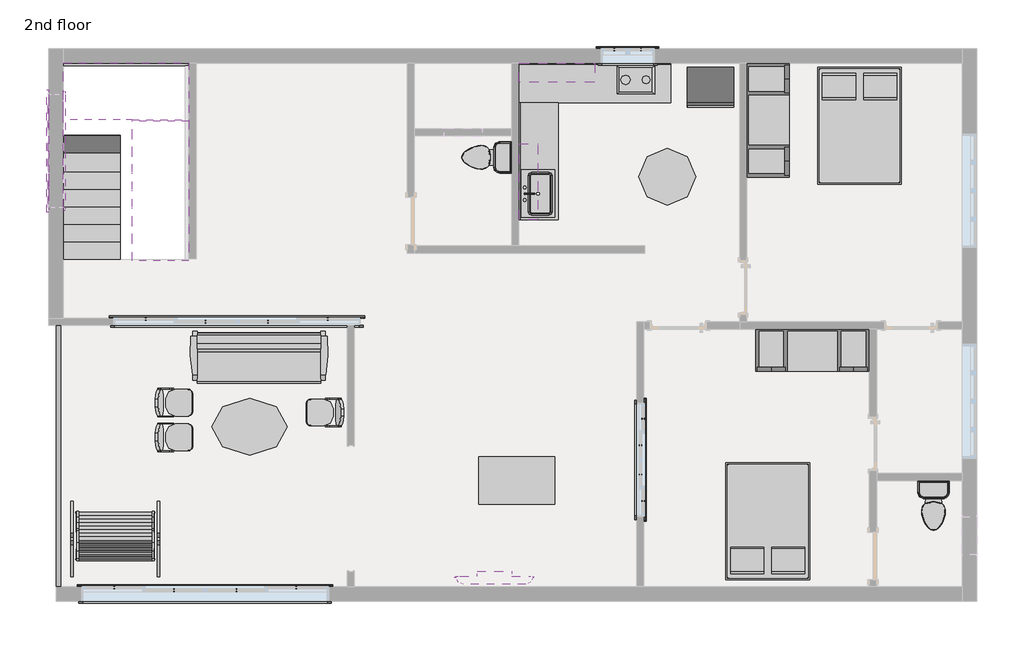
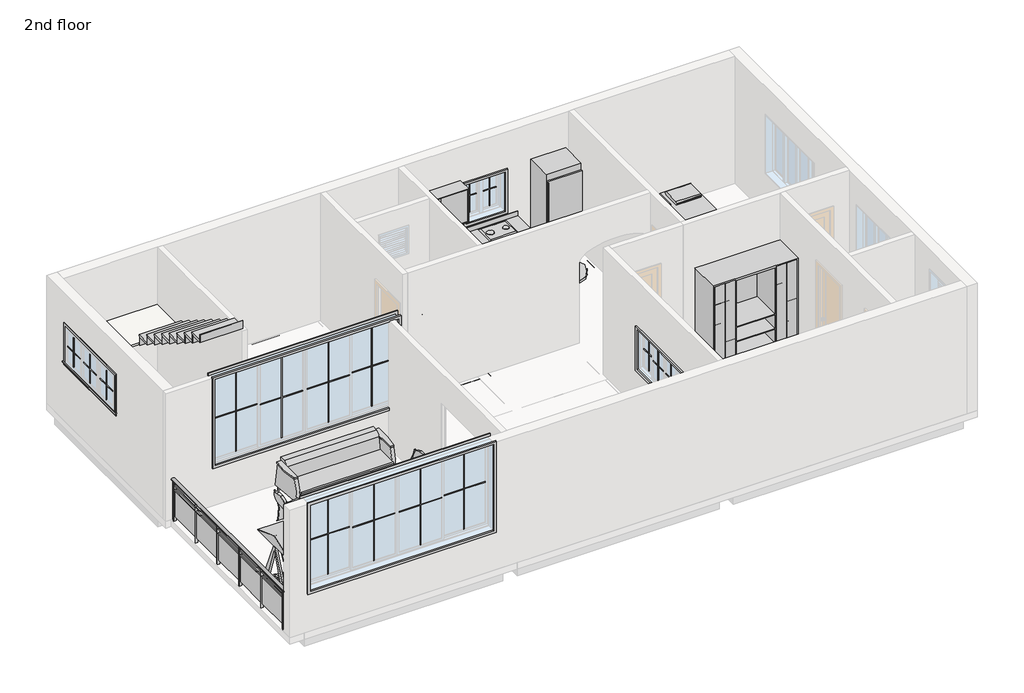
# One storey, part 2 of 2: 30 proxies, 21 furniture elements, 7 beams, 3 flow terminals, 2 stair flights, 1 railing, 1 slab.
"""IFC4 building model written with IfcOpenShell, lengths in millimetres."""

from ifc_helpers import new_model, si_unit, point, frame, origin, place, context, project, spatial, polyline, ellipse_curve, trimmed, outline, extrude, faceted_brep, transform, mapped, element, save
from ifc_brep_helpers import plane_surface, extruded_surface, advanced_brep
from components import proxy_3c1fa1d0, proxy_caef4acf, muntin_pattern_2x2_muntin_pattern_2x2_31a16349, muntin_pattern_2x2_muntin_pattern_2x2_a56fcb99, muntin_pattern_2x2_muntin_pattern_2x2_c58f38d7, muntin_pattern_2x2_muntin_pattern_2x2_b3fe6957, muntin_pattern_2x2_muntin_pattern_2x2_3e0ecaf2, muntin_pattern_2x2_muntin_pattern_2x2_51cb8927, proxy_19935bb1, trim_window_exterior_flat_with_sill_3c945769, trim_window_exterior_flat_with_sill_7b949e88, trim_window_exterior_flat_with_sill_41619996, trim_window_exterior_flat_with_sill_170b7f0e, trim_window_interior_flat_picture_frame_0edfbaa2, trim_window_interior_flat_picture_frame_687edbe0, trim_window_interior_flat_picture_frame_51c85655, trim_window_interior_flat_picture_frame_cc79b2fe, flow_terminal_4d548711, toilet_domestic_3d_toilet_domestic_3d_ba6479b0, toilet_domestic_3d_toilet_domestic_3d_30431060, furniture_0762_x_0762mm_a8fad5e2, furniture_f87f75a4, furniture_97fe820d, furniture_b58f7881, furniture_deb1c5d1, furniture_078eb3f3, furniture_88072bd9, furniture_eb3a3c23, furniture_4a9d42a7, furniture_0b81fedb, furniture_acc2807d, furniture_52f35bf4, furniture_b94c68a7, furniture_f491f192, non_monolithic_landing_4d8e9abd, stair_flight_485682bc, stair_flight_0c18b218

model = new_model("IFC4")

# Units and contexts
model_context = context("Model", 3, world=origin())
ifc_project = project(units=[si_unit("LENGTHUNIT", "METRE", prefix="MILLI")], contexts=[model_context])

# Site, building, storey
site = spatial("IfcSite", under=ifc_project)
building = spatial("IfcBuilding", under=site)
storey = spatial("IfcBuildingStorey", under=building, Name="2nd floor", Elevation=7010.4)

# Beams
placement = place(None, origin())
element("IfcBeam", 1, ObjectType="Concrete-Rectangular Beam", at=placement, inside=storey, context=model_context, shape_type="Brep", body=[
    faceted_brep([(-12643.368339, 9510.993496, 7010.4), (-12643.368339, 9282.393496, 7010.4), (-10681.218339, 9282.393496, 7010.4), (-10452.618339, 9282.393496, 7010.4), (-7176.018339, 9282.393496, 7010.4), (-6947.418339, 9282.393496, 7010.4), (-5499.618339, 9282.393496, 7010.4), (-5271.018339, 9282.393496, 7010.4), (-3492.916739, 9282.393496, 7010.4), (-3264.316739, 9282.393496, 7010.4), (-1842.018339, 9282.393496, 7010.4), (-1613.418339, 9282.393496, 7010.4), (1790.181661, 9282.393496, 7010.4), (1790.181661, 9510.993496, 7010.4), (-1575.318339, 9510.993496, 7010.4), (-1575.318339, 9320.493496, 7010.4), (-1880.118339, 9320.493496, 7010.4), (-1880.118339, 9510.993496, 7010.4), (-6909.318339, 9510.993496, 7010.4), (-6909.318339, 9320.493496, 7010.4), (-7214.118339, 9320.493496, 7010.4), (-7214.118339, 9510.993496, 7010.4), (-10414.518339, 9510.993496, 7010.4), (-10414.518339, 9320.493496, 7010.4), (-10719.318339, 9320.493496, 7010.4), (-10719.318339, 9510.993496, 7010.4), (-12643.368339, 9282.393496, 6705.6), (-10681.218339, 9282.393496, 6705.6), (-10452.618339, 9282.393496, 6705.6), (-7176.018339, 9282.393496, 6705.6), (-6947.418339, 9282.393496, 6705.6), (-5499.618339, 9282.393496, 6705.6), (-5271.018339, 9282.393496, 6705.6), (-3492.916739, 9282.393496, 6705.6), (-3264.316739, 9282.393496, 6705.6), (-1842.018339, 9282.393496, 6705.6), (-1613.418339, 9282.393496, 6705.6), (1790.181661, 9282.393496, 6705.6), (-12643.368339, 9510.993496, 6705.6), (-10719.318339, 9510.993496, 6705.6), (-10719.318339, 9320.493496, 6705.6), (-10414.518339, 9320.493496, 6705.6), (-10414.518339, 9510.993496, 6705.6), (-7214.118339, 9510.993496, 6705.6), (-7214.118339, 9320.493496, 6705.6), (-6909.318339, 9320.493496, 6705.6), (-6909.318339, 9510.993496, 6705.6), (-1880.118339, 9510.993496, 6705.6), (-1880.118339, 9320.493496, 6705.6), (-1575.318339, 9320.493496, 6705.6), (-1575.318339, 9510.993496, 6705.6), (1790.181661, 9510.993496, 6705.6)], [[[0, 1, 2, 3, 4, 5, 6, 7, 8, 9, 10, 11, 12, 13, 14, 15, 16, 17, 18, 19, 20, 21, 22, 23, 24, 25]], [[1, 26, 27, 28, 29, 30, 31, 32, 33, 34, 35, 36, 37, 12, 11, 10, 9, 8, 7, 6, 5, 4, 3, 2]], [[26, 38, 39, 40, 41, 42, 43, 44, 45, 46, 47, 48, 49, 50, 51, 37, 36, 35, 34, 33, 32, 31, 30, 29, 28, 27]], [[13, 51, 50, 14]], [[1, 0, 38, 26]], [[13, 12, 37, 51]], [[41, 23, 22, 42]], [[23, 41, 40, 24]], [[24, 40, 39, 25]], [[38, 0, 25, 39]], [[45, 19, 18, 46]], [[19, 45, 44, 20]], [[20, 44, 43, 21]], [[42, 22, 21, 43]], [[49, 15, 14, 50]], [[15, 49, 48, 16]], [[16, 48, 47, 17]], [[46, 18, 17, 47]]]),
])
element("IfcBeam", 2, ObjectType="Concrete-Rectangular Beam", at=placement, inside=storey, context=model_context, shape_type="Brep", body=[
    faceted_brep([(1790.181661, 913.093496, 7010.4), (2018.781661, 913.093496, 7010.4), (2018.781661, 4958.043496, 7010.4), (1790.181661, 4958.043496, 7010.4), (1790.181661, 2792.693496, 7010.4), (1790.181661, 2564.093496, 7010.4), (1790.181661, 913.093496, 6705.6), (1790.181661, 4958.043496, 6705.6), (1790.181661, 2792.693496, 6705.6), (1790.181661, 2564.093496, 6705.6), (2018.781661, 913.093496, 6705.6), (2018.781661, 4958.043496, 6705.6)], [[[0, 1, 2, 3, 4, 5]], [[6, 0, 5, 4, 3, 7, 8, 9]], [[10, 6, 9, 8, 7, 11]], [[1, 10, 11, 2]], [[1, 0, 6, 10]], [[3, 2, 11, 7]]]),
    faceted_brep([(1790.181661, 9244.293496, 7010.4), (2018.781661, 9244.293496, 7010.4), (2018.781661, 9244.293496, 6705.6), (1790.181661, 9244.293496, 6705.6), (2018.781661, 5262.843496, 7010.4), (1790.181661, 5262.843496, 7010.4), (1790.181661, 5262.843496, 6705.6), (2018.781661, 5262.843496, 6705.6), (1790.181661, 6289.4504179, 7010.4), (1790.181661, 6060.8155957, 7010.4), (1790.181661, 6289.4504179, 6705.6), (1790.181661, 6060.8155957, 6705.6)], [[[0, 1, 2, 3]], [[4, 5, 6, 7]], [[1, 0, 8, 9, 5, 4]], [[0, 3, 10, 11, 6, 5, 9, 8]], [[3, 2, 7, 6, 11, 10]], [[2, 1, 4, 7]]]),
])
element("IfcBeam", 3, ObjectType="Concrete-Rectangular Beam", at=placement, inside=storey, context=model_context, shape_type="SweptSolid", body=[
    extrude(outline(polyline([(-6947.418339, 8094.943496), (-6947.418339, 8323.543496), (-5499.618339, 8323.543496), (-5499.618339, 8094.943496), (-6947.418339, 8094.943496)])), frame((0.0, 0.0, 6705.6), z_axis=(0.0, 0.0, 1.0), x_axis=(1.0, 0.0, 0.0)), (0.0, 0.0, 1.0), 304.8),
])
element("IfcBeam", 4, ObjectType="Concrete-Rectangular Beam", at=placement, inside=storey, context=model_context, shape_type="Brep", body=[
    faceted_brep([(1790.181661, 6060.8155957, 7010.4), (1790.181661, 6289.4504179, 7010.4), (-1613.418339, 6348.8604768, 7010.4), (-1842.018339, 6352.8507047, 7010.4), (-3264.316739, 6377.6770156, 7010.4), (-3492.916739, 6381.6672435, 7010.4), (-5271.018339, 6412.7041223, 7010.4), (-5271.018339, 6184.0693001, 7010.4), (-3492.916739, 6153.0324213, 7010.4), (-3264.316739, 6149.0421934, 7010.4), (-1842.018339, 6124.2158825, 7010.4), (-1613.418339, 6120.2256547, 7010.4), (1790.181661, 6060.8155957, 6705.6), (-5271.018339, 6184.0693001, 6705.6), (-3492.916739, 6153.0324213, 6705.6), (-3264.316739, 6149.0421934, 6705.6), (-1842.018339, 6124.2158825, 6705.6), (-1613.418339, 6120.2256547, 6705.6), (1790.181661, 6289.4504179, 6705.6), (-5271.018339, 6412.7041223, 6705.6), (-3492.916739, 6381.6672435, 6705.6), (-3264.316739, 6377.6770156, 6705.6), (-1842.018339, 6352.8507047, 6705.6), (-1613.418339, 6348.8604768, 6705.6)], [[[0, 1, 2, 3, 4, 5, 6, 7, 8, 9, 10, 11]], [[12, 0, 11, 10, 9, 8, 7, 13, 14, 15, 16, 17]], [[18, 12, 17, 16, 15, 14, 13, 19, 20, 21, 22, 23]], [[1, 18, 23, 22, 21, 20, 19, 6, 5, 4, 3, 2]], [[1, 0, 12, 18]], [[7, 6, 19, 13]]]),
    faceted_brep([(-6947.418339, 6213.330971, 7010.4), (-6947.418339, 6441.9657932, 7010.4), (-6947.418339, 6441.9657932, 6705.6), (-6947.418339, 6213.330971, 6705.6), (-5499.618339, 6416.6943502, 7010.4), (-5499.618339, 6188.059528, 7010.4), (-5499.618339, 6188.059528, 6705.6), (-5499.618339, 6416.6943502, 6705.6)], [[[0, 1, 2, 3]], [[4, 5, 6, 7]], [[1, 0, 5, 4]], [[0, 3, 6, 5]], [[3, 2, 7, 6]], [[2, 1, 4, 7]]]),
])
element("IfcBeam", 5, ObjectType="Concrete-Rectangular Beam", at=placement, inside=storey, context=model_context, shape_type="Brep", body=[
    faceted_brep([(-1842.018339, 913.093496, 7010.4), (-1613.418339, 913.093496, 7010.4), (-1613.418339, 4996.143496, 7010.4), (-1613.418339, 5224.743496, 7010.4), (-1613.418339, 6120.2256547, 7010.4), (-1842.018339, 6124.2158825, 7010.4), (-1842.018339, 5281.893496, 7010.4), (-1784.868339, 5281.893496, 7010.4), (-1784.868339, 5053.293496, 7010.4), (-1842.018339, 5053.293496, 7010.4), (-1842.018339, 4996.143496, 7010.4), (-1842.018339, 913.093496, 6705.6), (-1842.018339, 5053.293496, 6705.6), (-1842.018339, 4996.143496, 6705.6), (-1613.418339, 913.093496, 6705.6), (-1784.868339, 5053.293496, 6705.6), (-1784.868339, 5281.893496, 6705.6), (-1842.018339, 5281.893496, 6705.6), (-1842.018339, 6124.2158825, 6705.6), (-1613.418339, 6120.2256547, 6705.6), (-1613.418339, 5224.743496, 6705.6), (-1613.418339, 4996.143496, 6705.6)], [[[0, 1, 2, 3, 4, 5, 6, 7, 8, 9, 10]], [[11, 0, 10, 9, 12, 13]], [[14, 11, 13, 12, 15, 16, 17, 18, 19, 20, 21]], [[1, 14, 21, 20, 19, 4, 3, 2]], [[1, 0, 11, 14]], [[5, 4, 19, 18]], [[8, 15, 12, 9]], [[16, 7, 6, 17]], [[7, 16, 15, 8]], [[5, 18, 17, 6]]]),
    faceted_brep([(-1842.018339, 9282.393496, 7010.4), (-1613.418339, 9282.393496, 7010.4), (-1613.418339, 9282.393496, 6705.6), (-1842.018339, 9282.393496, 6705.6), (-1613.418339, 6348.8604768, 7010.4), (-1842.018339, 6352.8507047, 7010.4), (-1842.018339, 6352.8507047, 6705.6), (-1613.418339, 6348.8604768, 6705.6)], [[[0, 1, 2, 3]], [[4, 5, 6, 7]], [[1, 0, 5, 4]], [[3, 2, 7, 6]], [[2, 1, 4, 7]], [[0, 3, 6, 5]]]),
])
element("IfcBeam", 6, ObjectType="Concrete-Rectangular Beam", at=placement, inside=storey, context=model_context, shape_type="Brep", body=[
    faceted_brep([(240.781661, 913.093496, 7010.4), (469.381661, 913.093496, 7010.4), (469.381661, 2564.093496, 7010.4), (469.381661, 2792.693496, 7010.4), (469.381661, 4996.143496, 7010.4), (240.781661, 4996.143496, 7010.4), (469.381661, 913.093496, 6705.6), (469.381661, 2564.093496, 6705.6), (469.381661, 2792.693496, 6705.6), (469.381661, 4996.143496, 6705.6), (240.781661, 913.093496, 6705.6), (240.781661, 4996.143496, 6705.6)], [[[0, 1, 2, 3, 4, 5]], [[1, 6, 7, 8, 9, 4, 3, 2]], [[6, 10, 11, 9, 8, 7]], [[10, 0, 5, 11]], [[1, 0, 10, 6]], [[5, 4, 9, 11]]]),
])
element("IfcBeam", 7, ObjectType="Concrete-Rectangular Beam", at=placement, inside=storey, context=model_context, shape_type="SweptSolid", body=[
    extrude(outline(polyline([(1790.181661, 2792.693496), (1790.181661, 2564.093496), (469.381661, 2564.093496), (469.381661, 2792.693496), (1790.181661, 2792.693496)])), frame((0.0, 0.0, 6705.6), z_axis=(0.0, 0.0, 1.0), x_axis=(1.0, 0.0, 0.0)), (0.0, 0.0, 1.0), 304.8),
])

# Proxies
proxy_shape = proxy_3c1fa1d0(model_context)
element("IfcBuildingElementProxy", 8, Name="Cook Top-2 Unit : 12\" x 18\"", ObjectType="Cook Top-2 Unit : 12\" x 18\"", at=placement, inside=storey, context=model_context, shape_type="MappedRepresentation", body=[
    mapped(proxy_shape, transform((-3421.5185434, 8977.593496, 7010.4), x_axis=(0.0, 1.0, 0.0), y_axis=(-1.0, 0.0, 0.0), z_axis=(0.0, 0.0, 1.0))),
])
proxy_2_shape = proxy_caef4acf(model_context)
element("IfcBuildingElementProxy", 9, Name="Cook Top-2 Unit : 16\" x 22\"", ObjectType="Cook Top-2 Unit : 16\" x 22\"", at=placement, inside=storey, context=model_context, shape_type="MappedRepresentation", body=[
    mapped(proxy_2_shape, transform((-3370.7185434, 8977.593496, 7010.4), x_axis=(0.0, 1.0, 0.0), y_axis=(-1.0, 0.0, 0.0), z_axis=(0.0, 0.0, 1.0))),
])
muntin_pattern_2x2_muntin_pattern_2x2_shape = muntin_pattern_2x2_muntin_pattern_2x2_31a16349(model_context)
element("IfcBuildingElementProxy", 10, Name="Muntin Pattern_2x2 : Muntin Pattern_2x2", ObjectType="Muntin Pattern_2x2 : Muntin Pattern_2x2", at=placement, inside=storey, context=model_context, shape_type="MappedRepresentation", body=[
    mapped(muntin_pattern_2x2_muntin_pattern_2x2_shape, transform((-3330.991739, 3615.018496, 8007.35), x_axis=(0.0, -1.0, 0.0), y_axis=(1.0, 0.0, 0.0), z_axis=(0.0, 0.0, 1.0))),
])
element("IfcBuildingElementProxy", 11, Name="Muntin Pattern_2x2 : Muntin Pattern_2x2", ObjectType="Muntin Pattern_2x2 : Muntin Pattern_2x2", at=placement, inside=storey, context=model_context, shape_type="MappedRepresentation", body=[
    mapped(muntin_pattern_2x2_muntin_pattern_2x2_shape, transform((-3375.441739, 3189.568496, 8007.35), x_axis=(0.0, -1.0, 0.0), y_axis=(1.0, 0.0, 0.0), z_axis=(0.0, 0.0, 1.0))),
])
element("IfcBuildingElementProxy", 12, Name="Muntin Pattern_2x2 : Muntin Pattern_2x2", ObjectType="Muntin Pattern_2x2 : Muntin Pattern_2x2", at=placement, inside=storey, context=model_context, shape_type="MappedRepresentation", body=[
    mapped(muntin_pattern_2x2_muntin_pattern_2x2_shape, transform((-3375.441739, 2719.668496, 8007.35), x_axis=(0.0, -1.0, 0.0), y_axis=(1.0, 0.0, 0.0), z_axis=(0.0, 0.0, 1.0))),
])
element("IfcBuildingElementProxy", 13, Name="Muntin Pattern_2x2 : Muntin Pattern_2x2", ObjectType="Muntin Pattern_2x2 : Muntin Pattern_2x2", at=placement, inside=storey, context=model_context, shape_type="MappedRepresentation", body=[
    mapped(muntin_pattern_2x2_muntin_pattern_2x2_shape, transform((-3330.991739, 2294.218496, 8007.35), x_axis=(0.0, -1.0, 0.0), y_axis=(1.0, 0.0, 0.0), z_axis=(0.0, 0.0, 1.0))),
])
muntin_pattern_2x2_muntin_pattern_2x2_2_shape = muntin_pattern_2x2_muntin_pattern_2x2_a56fcb99(model_context)
element("IfcBuildingElementProxy", 14, Name="Muntin Pattern_2x2 : Muntin Pattern_2x2", ObjectType="Muntin Pattern_2x2 : Muntin Pattern_2x2", at=placement, inside=storey, context=model_context, shape_type="MappedRepresentation", body=[
    mapped(muntin_pattern_2x2_muntin_pattern_2x2_2_shape, transform((-12862.443339, 7303.3101627, 8451.85), x_axis=(0.0, 1.0, 0.0), y_axis=(-1.0, 0.0, 0.0), z_axis=(0.0, 0.0, 1.0))),
])
element("IfcBuildingElementProxy", 15, Name="Muntin Pattern_2x2 : Muntin Pattern_2x2", ObjectType="Muntin Pattern_2x2 : Muntin Pattern_2x2", at=placement, inside=storey, context=model_context, shape_type="MappedRepresentation", body=[
    mapped(muntin_pattern_2x2_muntin_pattern_2x2_2_shape, transform((-12862.443339, 7910.793496, 8451.85), x_axis=(0.0, 1.0, 0.0), y_axis=(-1.0, 0.0, 0.0), z_axis=(0.0, 0.0, 1.0))),
])
muntin_pattern_2x2_muntin_pattern_2x2_3_shape = muntin_pattern_2x2_muntin_pattern_2x2_c58f38d7(model_context)
element("IfcBuildingElementProxy", 16, Name="Muntin Pattern_2x2 : Muntin Pattern_2x2", ObjectType="Muntin Pattern_2x2 : Muntin Pattern_2x2", at=placement, inside=storey, context=model_context, shape_type="MappedRepresentation", body=[
    mapped(muntin_pattern_2x2_muntin_pattern_2x2_3_shape, transform((-12862.443339, 8518.2768293, 8451.85), x_axis=(0.0, -1.0, 0.0), y_axis=(1.0, 0.0, 0.0), z_axis=(0.0, 0.0, 1.0))),
])
muntin_pattern_2x2_muntin_pattern_2x2_4_shape = muntin_pattern_2x2_muntin_pattern_2x2_b3fe6957(model_context)
element("IfcBuildingElementProxy", 17, Name="Muntin Pattern_2x2 : Muntin Pattern_2x2", ObjectType="Muntin Pattern_2x2 : Muntin Pattern_2x2", at=placement, inside=storey, context=model_context, shape_type="MappedRepresentation", body=[
    mapped(muntin_pattern_2x2_muntin_pattern_2x2_4_shape, transform((-3796.230839, 9539.568496, 8185.15), x_axis=(1.0, 0.0, 0.0), y_axis=(0.0, 1.0, 0.0), z_axis=(0.0, 0.0, 1.0))),
])
muntin_pattern_2x2_muntin_pattern_2x2_5_shape = muntin_pattern_2x2_muntin_pattern_2x2_3e0ecaf2(model_context)
element("IfcBuildingElementProxy", 18, Name="Muntin Pattern_2x2 : Muntin Pattern_2x2", ObjectType="Muntin Pattern_2x2 : Muntin Pattern_2x2", at=placement, inside=storey, context=model_context, shape_type="MappedRepresentation", body=[
    mapped(muntin_pattern_2x2_muntin_pattern_2x2_5_shape, transform((-3367.605839, 9539.568496, 8185.15), x_axis=(-1.0, 0.0, 0.0), y_axis=(0.0, -1.0, 0.0), z_axis=(0.0, 0.0, 1.0))),
])
muntin_pattern_2x2_muntin_pattern_2x2_6_shape = muntin_pattern_2x2_muntin_pattern_2x2_51cb8927(model_context)
element("IfcBuildingElementProxy", 19, Name="Muntin Pattern_2x2 : Muntin Pattern_2x2", ObjectType="Muntin Pattern_2x2 : Muntin Pattern_2x2", at=placement, inside=storey, context=model_context, shape_type="MappedRepresentation", body=[
    mapped(muntin_pattern_2x2_muntin_pattern_2x2_6_shape, transform((-11316.218339, 5215.218496, 8007.35), x_axis=(1.0, 0.0, 0.0), y_axis=(0.0, 1.0, 0.0), z_axis=(0.0, 0.0, 1.0))),
])
element("IfcBuildingElementProxy", 20, Name="Muntin Pattern_2x2 : Muntin Pattern_2x2", ObjectType="Muntin Pattern_2x2 : Muntin Pattern_2x2", at=placement, inside=storey, context=model_context, shape_type="MappedRepresentation", body=[
    mapped(muntin_pattern_2x2_muntin_pattern_2x2_6_shape, transform((-10357.368339, 5170.768496, 8007.35), x_axis=(1.0, 0.0, 0.0), y_axis=(0.0, 1.0, 0.0), z_axis=(0.0, 0.0, 1.0))),
])
element("IfcBuildingElementProxy", 21, Name="Muntin Pattern_2x2 : Muntin Pattern_2x2", ObjectType="Muntin Pattern_2x2 : Muntin Pattern_2x2", at=placement, inside=storey, context=model_context, shape_type="MappedRepresentation", body=[
    mapped(muntin_pattern_2x2_muntin_pattern_2x2_6_shape, transform((-9354.068339, 5170.768496, 8007.35), x_axis=(1.0, 0.0, 0.0), y_axis=(0.0, 1.0, 0.0), z_axis=(0.0, 0.0, 1.0))),
])
element("IfcBuildingElementProxy", 22, Name="Muntin Pattern_2x2 : Muntin Pattern_2x2", ObjectType="Muntin Pattern_2x2 : Muntin Pattern_2x2", at=placement, inside=storey, context=model_context, shape_type="MappedRepresentation", body=[
    mapped(muntin_pattern_2x2_muntin_pattern_2x2_6_shape, transform((-8395.218339, 5215.218496, 8007.35), x_axis=(1.0, 0.0, 0.0), y_axis=(0.0, 1.0, 0.0), z_axis=(0.0, 0.0, 1.0))),
])
element("IfcBuildingElementProxy", 23, Name="Muntin Pattern_2x2 : Muntin Pattern_2x2", ObjectType="Muntin Pattern_2x2 : Muntin Pattern_2x2", at=placement, inside=storey, context=model_context, shape_type="MappedRepresentation", body=[
    mapped(muntin_pattern_2x2_muntin_pattern_2x2_6_shape, transform((-11824.218339, 903.568496, 8007.35), x_axis=(1.0, 0.0, 0.0), y_axis=(0.0, 1.0, 0.0), z_axis=(0.0, 0.0, 1.0))),
])
element("IfcBuildingElementProxy", 24, Name="Muntin Pattern_2x2 : Muntin Pattern_2x2", ObjectType="Muntin Pattern_2x2 : Muntin Pattern_2x2", at=placement, inside=storey, context=model_context, shape_type="MappedRepresentation", body=[
    mapped(muntin_pattern_2x2_muntin_pattern_2x2_6_shape, transform((-10865.368339, 859.118496, 8007.35), x_axis=(1.0, 0.0, 0.0), y_axis=(0.0, 1.0, 0.0), z_axis=(0.0, 0.0, 1.0))),
])
element("IfcBuildingElementProxy", 25, Name="Muntin Pattern_2x2 : Muntin Pattern_2x2", ObjectType="Muntin Pattern_2x2 : Muntin Pattern_2x2", at=placement, inside=storey, context=model_context, shape_type="MappedRepresentation", body=[
    mapped(muntin_pattern_2x2_muntin_pattern_2x2_6_shape, transform((-9862.068339, 859.118496, 8007.35), x_axis=(1.0, 0.0, 0.0), y_axis=(0.0, 1.0, 0.0), z_axis=(0.0, 0.0, 1.0))),
])
element("IfcBuildingElementProxy", 26, Name="Muntin Pattern_2x2 : Muntin Pattern_2x2", ObjectType="Muntin Pattern_2x2 : Muntin Pattern_2x2", at=placement, inside=storey, context=model_context, shape_type="MappedRepresentation", body=[
    mapped(muntin_pattern_2x2_muntin_pattern_2x2_6_shape, transform((-8903.218339, 903.568496, 8007.35), x_axis=(1.0, 0.0, 0.0), y_axis=(0.0, 1.0, 0.0), z_axis=(0.0, 0.0, 1.0))),
])
proxy_3_shape = proxy_19935bb1(model_context)
element("IfcBuildingElementProxy", 27, Name="Refrigerator-Built-in : 30\" x 24\" LH", ObjectType="Refrigerator-Built-in : 30\" x 24\" LH", at=placement, inside=storey, context=model_context, shape_type="MappedRepresentation", body=[
    mapped(proxy_3_shape, transform((-2254.768339, 8966.8695245, 7010.4), x_axis=(1.0, 0.0, 0.0), y_axis=(0.0, 1.0, 0.0), z_axis=(0.0, 0.0, 1.0))),
])
trim_window_exterior_flat_with_sill_shape = trim_window_exterior_flat_with_sill_3c945769(model_context)
element("IfcBuildingElementProxy", 28, Name="Trim-Window-Exterior-Flat : with Sill", ObjectType="Trim-Window-Exterior-Flat : with Sill", at=placement, inside=storey, context=model_context, shape_type="MappedRepresentation", body=[
    mapped(trim_window_exterior_flat_with_sill_shape, transform((-3321.466739, 2954.618496, 8839.2), x_axis=(0.0, 1.0, 0.0), y_axis=(0.0, 0.0, 1.0), z_axis=(1.0, 0.0, 0.0))),
])
trim_window_exterior_flat_with_sill_2_shape = trim_window_exterior_flat_with_sill_7b949e88(model_context)
element("IfcBuildingElementProxy", 29, Name="Trim-Window-Exterior-Flat : with Sill", ObjectType="Trim-Window-Exterior-Flat : with Sill", at=placement, inside=storey, context=model_context, shape_type="MappedRepresentation", body=[
    mapped(trim_window_exterior_flat_with_sill_2_shape, transform((-12871.968339, 7910.793496, 9194.8), x_axis=(0.0, 1.0, 0.0), y_axis=(0.0, 0.0, -1.0), z_axis=(-1.0, 0.0, 0.0))),
])
trim_window_exterior_flat_with_sill_3_shape = trim_window_exterior_flat_with_sill_41619996(model_context)
element("IfcBuildingElementProxy", 30, Name="Trim-Window-Exterior-Flat : with Sill", ObjectType="Trim-Window-Exterior-Flat : with Sill", at=placement, inside=storey, context=model_context, shape_type="MappedRepresentation", body=[
    mapped(trim_window_exterior_flat_with_sill_3_shape, transform((-3581.918339, 9549.093496, 9029.7), x_axis=(-1.0, 0.0, 0.0), y_axis=(0.0, 0.0, 1.0), z_axis=(0.0, 1.0, 0.0))),
])
trim_window_exterior_flat_with_sill_4_shape = trim_window_exterior_flat_with_sill_170b7f0e(model_context)
element("IfcBuildingElementProxy", 31, Name="Trim-Window-Exterior-Flat : with Sill", ObjectType="Trim-Window-Exterior-Flat : with Sill", at=placement, inside=storey, context=model_context, shape_type="MappedRepresentation", body=[
    mapped(trim_window_exterior_flat_with_sill_4_shape, transform((-9855.718339, 5224.743496, 9906.0), x_axis=(-1.0, 0.0, 0.0), y_axis=(0.0, 0.0, 1.0), z_axis=(0.0, 1.0, 0.0))),
])
element("IfcBuildingElementProxy", 32, Name="Trim-Window-Exterior-Flat : with Sill", ObjectType="Trim-Window-Exterior-Flat : with Sill", at=placement, inside=storey, context=model_context, shape_type="MappedRepresentation", body=[
    mapped(trim_window_exterior_flat_with_sill_4_shape, transform((-10363.718339, 913.093496, 9906.0), x_axis=(-1.0, 0.0, 0.0), y_axis=(0.0, 0.0, 1.0), z_axis=(0.0, 1.0, 0.0))),
])
trim_window_interior_flat_picture_frame_shape = trim_window_interior_flat_picture_frame_0edfbaa2(model_context)
element("IfcBuildingElementProxy", 33, Name="Trim-Window-Interior-Flat : Picture Frame", ObjectType="Trim-Window-Interior-Flat : Picture Frame", at=placement, inside=storey, context=model_context, shape_type="MappedRepresentation", body=[
    mapped(trim_window_interior_flat_picture_frame_shape, transform((-3435.766739, 2954.618496, 8839.2), x_axis=(0.0, -1.0, 0.0), y_axis=(0.0, 0.0, 1.0), z_axis=(-1.0, 0.0, 0.0))),
])
trim_window_interior_flat_picture_frame_2_shape = trim_window_interior_flat_picture_frame_687edbe0(model_context)
element("IfcBuildingElementProxy", 34, Name="Trim-Window-Interior-Flat : Picture Frame", ObjectType="Trim-Window-Interior-Flat : Picture Frame", at=placement, inside=storey, context=model_context, shape_type="MappedRepresentation", body=[
    mapped(trim_window_interior_flat_picture_frame_2_shape, transform((-12643.368339, 7910.793496, 9194.8), x_axis=(0.0, -1.0, 0.0), y_axis=(0.0, 0.0, -1.0), z_axis=(1.0, 0.0, 0.0))),
])
trim_window_interior_flat_picture_frame_3_shape = trim_window_interior_flat_picture_frame_51c85655(model_context)
element("IfcBuildingElementProxy", 35, Name="Trim-Window-Interior-Flat : Picture Frame", ObjectType="Trim-Window-Interior-Flat : Picture Frame", at=placement, inside=storey, context=model_context, shape_type="MappedRepresentation", body=[
    mapped(trim_window_interior_flat_picture_frame_3_shape, transform((-3581.918339, 9320.493496, 9029.7), x_axis=(1.0, 0.0, 0.0), y_axis=(0.0, 0.0, 1.0), z_axis=(0.0, -1.0, 0.0))),
])
trim_window_interior_flat_picture_frame_4_shape = trim_window_interior_flat_picture_frame_cc79b2fe(model_context)
element("IfcBuildingElementProxy", 36, Name="Trim-Window-Interior-Flat : Picture Frame", ObjectType="Trim-Window-Interior-Flat : Picture Frame", at=placement, inside=storey, context=model_context, shape_type="MappedRepresentation", body=[
    mapped(trim_window_interior_flat_picture_frame_4_shape, transform((-9855.718339, 5110.443496, 9906.0), x_axis=(1.0, 0.0, 0.0), y_axis=(0.0, 0.0, 1.0), z_axis=(0.0, -1.0, 0.0))),
])
element("IfcBuildingElementProxy", 37, Name="Trim-Window-Interior-Flat : Picture Frame", ObjectType="Trim-Window-Interior-Flat : Picture Frame", at=placement, inside=storey, context=model_context, shape_type="MappedRepresentation", body=[
    mapped(trim_window_interior_flat_picture_frame_4_shape, transform((-10363.718339, 684.493496, 9906.0), x_axis=(1.0, 0.0, 0.0), y_axis=(0.0, 0.0, 1.0), z_axis=(0.0, -1.0, 0.0))),
])

# Flow terminals
flow_terminal_shape = flow_terminal_4d548711(model_context)
element("IfcFlowTerminal", 38, ObjectType="Sink Kitchen-Single : 30\" x 21\"", at=placement, inside=storey, context=model_context, shape_type="MappedRepresentation", body=[
    mapped(flow_terminal_shape, transform((-5021.0229378, 7209.3042554, 7010.4), x_axis=(0.0, 1.0, 0.0), y_axis=(-1.0, 0.0, 0.0), z_axis=(0.0, 0.0, 1.0))),
])
toilet_domestic_3d_toilet_domestic_3d_shape = toilet_domestic_3d_toilet_domestic_3d_ba6479b0(model_context)
toilet_domestic_3d_toilet_domestic_3d_2_shape = toilet_domestic_3d_toilet_domestic_3d_30431060(model_context)
element("IfcFlowTerminal", 39, ObjectType="Toilet-Domestic-3D : Toilet-Domestic-3D", at=placement, inside=storey, context=model_context, shape_type="MappedRepresentation", body=[
    mapped(toilet_domestic_3d_toilet_domestic_3d_shape, transform((-5937.1643663, 7809.6710196, 7010.4), x_axis=(0.0, -1.0, 0.0), y_axis=(1.0, 0.0, 0.0), z_axis=(0.0, 0.0, 1.0))),
    mapped(toilet_domestic_3d_toilet_domestic_3d_2_shape, transform((-5937.1643663, 7809.6710196, 7010.4), x_axis=(0.0, -1.0, 0.0), y_axis=(1.0, 0.0, 0.0), z_axis=(0.0, 0.0, 1.0))),
])
element("IfcFlowTerminal", 40, ObjectType="Toilet-Domestic-3D : Toilet-Domestic-3D", at=placement, inside=storey, context=model_context, shape_type="MappedRepresentation", body=[
    mapped(toilet_domestic_3d_toilet_domestic_3d_shape, transform((1325.531896, 2126.5474686, 7010.4), x_axis=(1.0, 0.0, 0.0), y_axis=(0.0, 1.0, 0.0), z_axis=(0.0, 0.0, 1.0))),
    mapped(toilet_domestic_3d_toilet_domestic_3d_2_shape, transform((1325.531896, 2126.5474686, 7010.4), x_axis=(1.0, 0.0, 0.0), y_axis=(0.0, 1.0, 0.0), z_axis=(0.0, 0.0, 1.0))),
])

# Furniture
furniture_0762_x_0762mm_shape = furniture_0762_x_0762mm_a8fad5e2(model_context)
element("IfcFurniture", 41, ObjectType="0762 x 0762mm", at=placement, inside=storey, context=model_context, shape_type="MappedRepresentation", body=[
    mapped(furniture_0762_x_0762mm_shape, transform((-11368.6588951, 2598.8675531, 7010.4), x_axis=(-1.0, 0.0, 0.0), y_axis=(0.0, -1.0, 0.0), z_axis=(0.0, 0.0, 1.0))),
])
furniture_shape = furniture_f87f75a4(model_context)
element("IfcFurniture", 42, ObjectType="Base Cabinet-Combo01 : 30\"", at=placement, inside=storey, context=model_context, shape_type="MappedRepresentation", body=[
    mapped(furniture_shape, transform((-4051.5060439, 9320.493496, 7010.4), x_axis=(1.0, 0.0, 0.0), y_axis=(0.0, 1.0, 0.0), z_axis=(0.0, 0.0, 1.0))),
])
element("IfcFurniture", 43, ObjectType="Base Cabinet-Combo01 : 30\"", at=placement, inside=storey, context=model_context, shape_type="MappedRepresentation", body=[
    mapped(furniture_shape, transform((-5328.168339, 8006.3557911, 7010.4), x_axis=(0.0, 1.0, 0.0), y_axis=(-1.0, 0.0, 0.0), z_axis=(0.0, 0.0, 1.0))),
])
element("IfcFurniture", 44, ObjectType="Base Cabinet-Combo01 : 30\"", at=placement, inside=storey, context=model_context, shape_type="MappedRepresentation", body=[
    mapped(furniture_shape, transform((-3289.5060439, 9320.493496, 7010.4), x_axis=(1.0, 0.0, 0.0), y_axis=(0.0, 1.0, 0.0), z_axis=(0.0, 0.0, 1.0))),
])
furniture_2_shape = furniture_97fe820d(model_context)
element("IfcFurniture", 45, ObjectType="Base Cabinet-Corner Unit-Square : 36\"", at=placement, inside=storey, context=model_context, shape_type="MappedRepresentation", body=[
    mapped(furniture_2_shape, transform((-5328.168339, 8793.7557911, 7010.4), x_axis=(0.0, 1.0, 0.0), y_axis=(-1.0, 0.0, 0.0), z_axis=(0.0, 0.0, 1.0))),
])
furniture_3_shape = furniture_b58f7881(model_context)
element("IfcFurniture", 46, ObjectType="Bed-Box : Double 53\" x 74\"", at=placement, inside=storey, context=model_context, shape_type="MappedRepresentation", body=[
    mapped(furniture_3_shape, transform((-199.970798, 8551.6230042, 7010.4), x_axis=(1.0, 0.0, 0.0), y_axis=(0.0, 1.0, 0.0), z_axis=(0.0, 0.0, 1.0))),
])
element("IfcFurniture", 47, ObjectType="Bed-Box : Double 53\" x 74\"", at=placement, inside=storey, context=model_context, shape_type="MappedRepresentation", body=[
    mapped(furniture_3_shape, transform((-994.7642799, 1732.7639878, 7010.4), x_axis=(-1.0, 0.0, 0.0), y_axis=(0.0, -1.0, 0.0), z_axis=(0.0, 0.0, 1.0))),
])
furniture_4_shape = furniture_deb1c5d1(model_context)
element("IfcFurniture", 48, ObjectType="Counter Top : 24\" Depth", at=placement, inside=storey, context=model_context, shape_type="MappedRepresentation", body=[
    mapped(furniture_4_shape, transform((-4127.7060439, 9320.493496, 7010.4), x_axis=(1.0, 0.0, 0.0), y_axis=(0.0, 1.0, 0.0), z_axis=(0.0, 0.0, 1.0))),
])
furniture_5_shape = furniture_078eb3f3(model_context)
element("IfcFurniture", 49, ObjectType="Counter Top w Sink Hole : 24\" Depth", at=placement, inside=storey, context=model_context, shape_type="MappedRepresentation", body=[
    mapped(furniture_5_shape, transform((-5328.168339, 8006.6364215, 7010.4), x_axis=(0.0, 1.0, 0.0), y_axis=(-1.0, 0.0, 0.0), z_axis=(0.0, 0.0, 1.0))),
])
furniture_6_shape = furniture_88072bd9(model_context)
element("IfcFurniture", 50, ObjectType="Entertainment Center.0001 : 72\" x 72\" x 24\"", at=placement, inside=storey, context=model_context, shape_type="MappedRepresentation", body=[
    mapped(furniture_6_shape, transform((-616.468339, 5154.893496, 7010.4), x_axis=(1.0, 0.0, 0.0), y_axis=(0.0, 1.0, 0.0), z_axis=(0.0, 0.0, 1.0))),
])
element("IfcFurniture", 51, ObjectType="Entertainment Center.0001 : 72\" x 72\" x 24\"", at=placement, inside=storey, context=model_context, shape_type="MappedRepresentation", body=[
    mapped(furniture_6_shape, transform((-1772.168339, 8406.093496, 7010.4), x_axis=(0.0, 1.0, 0.0), y_axis=(-1.0, 0.0, 0.0), z_axis=(0.0, 0.0, 1.0))),
])
furniture_7_shape = furniture_eb3a3c23(model_context)
element("IfcFurniture", 52, ObjectType="Seating-Auditorium : 18\" x 24\" x 30\"", at=placement, inside=storey, context=model_context, shape_type="MappedRepresentation", body=[
    mapped(furniture_7_shape, transform((-8243.4429291, 3552.7156271, 7010.4), x_axis=(0.0, 1.0, 0.0), y_axis=(-1.0, 0.0, 0.0), z_axis=(0.0, 0.0, 1.0))),
])
element("IfcFurniture", 53, ObjectType="Seating-Auditorium : 18\" x 24\" x 30\"", at=placement, inside=storey, context=model_context, shape_type="MappedRepresentation", body=[
    mapped(furniture_7_shape, transform((-11061.5937488, 3474.1213649, 7010.4), x_axis=(0.0, -1.0, 0.0), y_axis=(1.0, 0.0, 0.0), z_axis=(0.0, 0.0, 1.0))),
])
element("IfcFurniture", 54, ObjectType="Seating-Auditorium : 18\" x 24\" x 30\"", at=placement, inside=storey, context=model_context, shape_type="MappedRepresentation", body=[
    mapped(furniture_7_shape, transform((-11061.5937488, 4032.9213649, 7010.4), x_axis=(0.0, -1.0, 0.0), y_axis=(1.0, 0.0, 0.0), z_axis=(0.0, 0.0, 1.0))),
])
furniture_8_shape = furniture_4a9d42a7(model_context)
element("IfcFurniture", 55, ObjectType="Sofa-Pensi : 84\"", at=placement, inside=storey, context=model_context, shape_type="MappedRepresentation", body=[
    mapped(furniture_8_shape, transform((-9778.724589, 4325.3336599, 7010.4), x_axis=(1.0, 0.0, 0.0), y_axis=(0.0, 1.0, 0.0), z_axis=(0.0, 0.0, 1.0))),
])
furniture_9_shape = furniture_0b81fedb(model_context)
element("IfcFurniture", 56, ObjectType="TV - Flat Screen : 50\"", at=placement, inside=storey, context=model_context, shape_type="MappedRepresentation", body=[
    mapped(furniture_9_shape, transform((-5725.8128531, 1013.6142575, 8229.6), x_axis=(-1.0, 0.0, 0.0), y_axis=(0.0, -1.0, 0.0), z_axis=(0.0, 0.0, 1.0))),
])
furniture_10_shape = furniture_acc2807d(model_context)
element("IfcFurniture", 57, ObjectType="Table-Coffee Rectangular : 48\" x 30\"", at=placement, inside=storey, context=model_context, shape_type="MappedRepresentation", body=[
    mapped(furniture_10_shape, transform((-5973.1503692, 2251.6326642, 7010.4), x_axis=(1.0, 0.0, 0.0), y_axis=(0.0, 1.0, 0.0), z_axis=(0.0, 0.0, 1.0))),
])
furniture_11_shape = furniture_52f35bf4(model_context)
element("IfcFurniture", 58, ObjectType="Table-Dining Round w Chairs : 36\" Diameter", at=placement, inside=storey, context=model_context, shape_type="MappedRepresentation", body=[
    mapped(furniture_11_shape, transform((-3050.6003062, 7682.9221845, 7010.4), x_axis=(1.0, 0.0, 0.0), y_axis=(0.0, 1.0, 0.0), z_axis=(0.0, 0.0, 1.0))),
])
furniture_12_shape = furniture_b94c68a7(model_context)
element("IfcFurniture", 59, ObjectType="Table-Ellipse : 60\" x 48\"", at=placement, inside=storey, context=model_context, shape_type="MappedRepresentation", body=[
    mapped(furniture_12_shape, transform((-9652.518339, 3484.843496, 7010.4), x_axis=(1.0, 0.0, 0.0), y_axis=(0.0, 1.0, 0.0), z_axis=(0.0, 0.0, 1.0))),
])
furniture_13_shape = furniture_f491f192(model_context)
element("IfcFurniture", 60, ObjectType="Upper Cabinet-Pass-Thru w Glass : 48\" x 30\" x 12\"", at=placement, inside=storey, context=model_context, shape_type="MappedRepresentation", body=[
    mapped(furniture_13_shape, transform((-4737.3060439, 9320.493496, 7010.4), x_axis=(1.0, 0.0, 0.0), y_axis=(0.0, 1.0, 0.0), z_axis=(0.0, 0.0, 1.0))),
])
element("IfcFurniture", 61, ObjectType="Upper Cabinet-Pass-Thru w Glass : 48\" x 30\" x 12\"", at=placement, inside=storey, context=model_context, shape_type="MappedRepresentation", body=[
    mapped(furniture_13_shape, transform((-5328.168339, 7397.0364215, 7010.4), x_axis=(0.0, 1.0, 0.0), y_axis=(-1.0, 0.0, 0.0), z_axis=(0.0, 0.0, 1.0))),
])

# Railing
element("IfcRailing", 62, ObjectType="Glass Panel - Bottom Fill", at=placement, inside=storey, context=model_context, shape_type="SolidModel", body=[
    advanced_brep(
    [(-12681.468339, 5110.443496, 7924.8), (-12757.668339, 5110.443496, 7924.8), (-12681.468339, 913.093496, 7924.8), (-12757.668339, 913.093496, 7924.8)],
    [
        (0, 1, ellipse_curve(frame((-12719.568339, 5110.443496, 7924.8), z_axis=(0.0, 1.0, 0.0), x_axis=(-1.0, 0.0, 0.0)), 38.1, 28.575)),
        (1, 0, ellipse_curve(frame((-12719.568339, 5110.443496, 7924.8), z_axis=(0.0, 1.0, 0.0), x_axis=(-1.0, 0.0, 0.0)), 38.1, 28.575)),
        (2, 3, ellipse_curve(frame((-12719.568339, 913.093496, 7924.8), z_axis=(0.0, -1.0, 0.0), x_axis=(-1.0, 0.0, 0.0)), 38.1, 28.575)),
        (3, 2, ellipse_curve(frame((-12719.568339, 913.093496, 7924.8), z_axis=(0.0, -1.0, 0.0), x_axis=(-1.0, 0.0, 0.0)), 38.1, 28.575)),
        (0, 2),
        (3, 1),
    ],
    [
        plane_surface(frame((-12719.568339, 5110.443496, 7924.8), z_axis=(0.0, 1.0, 0.0), x_axis=(0.0, 0.0, -1.0))),
        plane_surface(frame((-12719.568339, 913.093496, 7924.8), z_axis=(0.0, -1.0, 0.0), x_axis=(0.0, 0.0, -1.0))),
        extruded_surface(trimmed(ellipse_curve(frame((-12719.568339, 913.093496, 7924.8), z_axis=(0.0, 1.0, 0.0), x_axis=(-1.0, 0.0, 0.0)), 38.1, 28.575), [point((-12681.468339, 913.093496, 7924.8))], [point((-12757.668339, 913.093496, 7924.8))], True, "CARTESIAN"), (0.0, 4197.35, 0.0), 4197.35),
        extruded_surface(trimmed(ellipse_curve(frame((-12719.568339, 913.093496, 7924.8), z_axis=(0.0, 1.0, 0.0), x_axis=(-1.0, 0.0, 0.0)), 38.1, 28.575), [point((-12757.668339, 913.093496, 7924.8))], [point((-12681.468339, 913.093496, 7924.8))], True, "CARTESIAN"), (0.0, 4197.35, 0.0), 4197.35),
    ],
    [
        (0, [[1, 2]]),
        (1, [[3, 4]]),
        (2, [[-1, 5, -4, 6]]),
        (3, [[-2, -6, -3, -5]]),
    ],
),
    extrude(outline(polyline([(-12732.268339, 5110.443496), (-12706.868339, 5110.443496), (-12706.868339, 913.093496), (-12732.268339, 913.093496), (-12732.268339, 5110.443496)])), frame((0.0, 0.0, 7810.5), z_axis=(0.0, 0.0, 1.0), x_axis=(1.0, 0.0, 0.0)), (0.0, 0.0, 1.0), 25.4),
    extrude(outline(polyline([(-12732.268339, 5110.443496), (-12706.868339, 5110.443496), (-12706.868339, 913.093496), (-12732.268339, 913.093496), (-12732.268339, 5110.443496)])), frame((0.0, 0.0, 7708.9), z_axis=(0.0, 0.0, 1.0), x_axis=(1.0, 0.0, 0.0)), (0.0, 0.0, 1.0), 25.4),
    extrude(outline(polyline([(-12744.968339, 986.118496), (-12694.168339, 986.118496), (-12694.168339, 973.418496), (-12744.968339, 973.418496), (-12744.968339, 986.118496)])), frame((0.0, 0.0, 7010.4), z_axis=(0.0, 0.0, 1.0), x_axis=(1.0, 0.0, 0.0)), (0.0, 0.0, 1.0), 885.825),
    extrude(outline(polyline([(-12713.0331819, 1792.568496), (-12713.0331819, 979.768496), (-12719.3831819, 979.768496), (-12719.3831819, 1792.568496), (-12713.0331819, 1792.568496)])), frame((0.0, 0.0, 7112.0), z_axis=(0.0, 0.0, 1.0), x_axis=(1.0, 0.0, 0.0)), (0.0, 0.0, 1.0), 596.9),
    extrude(outline(polyline([(-12744.968339, 1798.918496), (-12694.168339, 1798.918496), (-12694.168339, 1786.218496), (-12744.968339, 1786.218496), (-12744.968339, 1798.918496)])), frame((0.0, 0.0, 7010.4), z_axis=(0.0, 0.0, 1.0), x_axis=(1.0, 0.0, 0.0)), (0.0, 0.0, 1.0), 885.825),
    extrude(outline(polyline([(-12713.0331819, 2605.368496), (-12713.0331819, 1792.568496), (-12719.3831819, 1792.568496), (-12719.3831819, 2605.368496), (-12713.0331819, 2605.368496)])), frame((0.0, 0.0, 7112.0), z_axis=(0.0, 0.0, 1.0), x_axis=(1.0, 0.0, 0.0)), (0.0, 0.0, 1.0), 596.9),
    extrude(outline(polyline([(-12744.968339, 2611.718496), (-12694.168339, 2611.718496), (-12694.168339, 2599.018496), (-12744.968339, 2599.018496), (-12744.968339, 2611.718496)])), frame((0.0, 0.0, 7010.4), z_axis=(0.0, 0.0, 1.0), x_axis=(1.0, 0.0, 0.0)), (0.0, 0.0, 1.0), 885.825),
    extrude(outline(polyline([(-12713.0331819, 3418.168496), (-12713.0331819, 2605.368496), (-12719.3831819, 2605.368496), (-12719.3831819, 3418.168496), (-12713.0331819, 3418.168496)])), frame((0.0, 0.0, 7112.0), z_axis=(0.0, 0.0, 1.0), x_axis=(1.0, 0.0, 0.0)), (0.0, 0.0, 1.0), 596.9),
    extrude(outline(polyline([(-12744.968339, 3424.518496), (-12694.168339, 3424.518496), (-12694.168339, 3411.818496), (-12744.968339, 3411.818496), (-12744.968339, 3424.518496)])), frame((0.0, 0.0, 7010.4), z_axis=(0.0, 0.0, 1.0), x_axis=(1.0, 0.0, 0.0)), (0.0, 0.0, 1.0), 885.825),
    extrude(outline(polyline([(-12713.0331819, 4230.968496), (-12713.0331819, 3418.168496), (-12719.3831819, 3418.168496), (-12719.3831819, 4230.968496), (-12713.0331819, 4230.968496)])), frame((0.0, 0.0, 7112.0), z_axis=(0.0, 0.0, 1.0), x_axis=(1.0, 0.0, 0.0)), (0.0, 0.0, 1.0), 596.9),
    extrude(outline(polyline([(-12744.968339, 4237.318496), (-12694.168339, 4237.318496), (-12694.168339, 4224.618496), (-12744.968339, 4224.618496), (-12744.968339, 4237.318496)])), frame((0.0, 0.0, 7010.4), z_axis=(0.0, 0.0, 1.0), x_axis=(1.0, 0.0, 0.0)), (0.0, 0.0, 1.0), 885.825),
    extrude(outline(polyline([(-12713.0331819, 5043.768496), (-12713.0331819, 4230.968496), (-12719.3831819, 4230.968496), (-12719.3831819, 5043.768496), (-12713.0331819, 5043.768496)])), frame((0.0, 0.0, 7112.0), z_axis=(0.0, 0.0, 1.0), x_axis=(1.0, 0.0, 0.0)), (0.0, 0.0, 1.0), 596.9),
    extrude(outline(polyline([(-12744.968339, 5050.118496), (-12694.168339, 5050.118496), (-12694.168339, 5037.418496), (-12744.968339, 5037.418496), (-12744.968339, 5050.118496)])), frame((0.0, 0.0, 7010.4), z_axis=(0.0, 0.0, 1.0), x_axis=(1.0, 0.0, 0.0)), (0.0, 0.0, 1.0), 885.825),
    extrude(outline(polyline([(-12729.093339, 925.793496), (-12710.043339, 925.793496), (-12710.043339, 906.743496), (-12729.093339, 906.743496), (-12729.093339, 925.793496)])), frame((0.0, 0.0, 7010.4), z_axis=(0.0, 0.0, 1.0), x_axis=(1.0, 0.0, 0.0)), (0.0, 0.0, 1.0), 885.825),
    extrude(outline(polyline([(-12729.093339, 5116.793496), (-12710.043339, 5116.793496), (-12710.043339, 5097.743496), (-12729.093339, 5097.743496), (-12729.093339, 5116.793496)])), frame((0.0, 0.0, 7010.4), z_axis=(0.0, 0.0, 1.0), x_axis=(1.0, 0.0, 0.0)), (0.0, 0.0, 1.0), 885.825),
])

# Slab
non_monolithic_landing_shape = non_monolithic_landing_4d8e9abd(model_context)
element("IfcSlab", 63, ObjectType="Non-Monolithic Landing", at=placement, inside=storey, context=model_context, shape_type="MappedRepresentation", body=[
    mapped(non_monolithic_landing_shape, transform((0.0, 0.0, 0.0), x_axis=(1.0, 0.0, 0.0), y_axis=(0.0, 1.0, 0.0), z_axis=(0.0, 0.0, 1.0))),
])

# Stair flights
stair_flight_shape = stair_flight_485682bc(model_context)
element("IfcStairFlight", 64, ObjectType="2\" Tread 1\" Nosing 1/4\" Riser", at=placement, inside=storey, context=model_context, shape_type="MappedRepresentation", body=[
    mapped(stair_flight_shape, transform((0.0, 0.0, 0.0), x_axis=(1.0, 0.0, 0.0), y_axis=(0.0, 1.0, 0.0), z_axis=(0.0, 0.0, 1.0))),
])
stair_flight_2_shape = stair_flight_0c18b218(model_context)
element("IfcStairFlight", 65, ObjectType="2\" Tread 1\" Nosing 1/4\" Riser", at=placement, inside=storey, context=model_context, shape_type="MappedRepresentation", body=[
    mapped(stair_flight_2_shape, transform((0.0, 0.0, 0.0), x_axis=(1.0, 0.0, 0.0), y_axis=(0.0, 1.0, 0.0), z_axis=(0.0, 0.0, 1.0))),
])

save(model, "model.ifc")

# Revit data of these elements
# Type "Concrete-Rectangular Beam"
#   Assembly Code = "B10"
#   Length [instance default] = 5 ft
#   b = 0.75 ft
#   h = 1 ft
#   Structural Material [instance default] = Concrete, Cast-in-Place gray
# Type "Cook Top-2 Unit : 12\" x 18\""
#   Assembly Code = "E1090400"
#   Counter Height = 3 ft
#   Depth = 2 ft
#   Width = 1.5 ft
#   Burner Material = Metal - Chrome
#   Cooktop Material = Metal - Steel, Polished
#   Default Elevation = 0
# Type "Cook Top-2 Unit : 16\" x 22\""
#   Assembly Code = "E1090400"
#   Counter Height = 2.583333 ft
#   Depth = 1.833333 ft
#   Width = 1.333333 ft
#   Burner Material = Metal - Chrome
#   Cooktop Material = Metal - Steel, Polished
#   Default Elevation = 0
# Type "Muntin Pattern_2x2 : Muntin Pattern_2x2"
#   Width [instance default] = 4 ft
#   Thickness = 0.041667 ft
#   Height [instance default] = 4 ft
#   Distance = 0.0625 ft
#   Interior Material [instance default] = none
#   Exterior Material [instance default] = none
#   Default Elevation = 0
# Type "Refrigerator-Built-in : 30\" x 24\" LH"
#   Assembly Code = "E1090400"
#   Depth = 2 ft
#   Handle = 0.020833 ft
#   Height = 7 ft
#   Top Door Height = 5 ft
#   Width = 2.458333 ft
#   Material = Metal - Paint Finish - Ivory,Glossy
#   Default Elevation = 0
# Type "Trim-Window-Exterior-Flat : with Sill"
#   Trim Width = 0.1875 ft
#   Trim Thickness_Picture Frame = 0.104167 ft
#   Trim Thickness_with Sill = 0.0625 ft
#   Sill Thickness = 0.104167 ft
#   Opening Width [instance default] = 2 ft
#   Opening Height [instance default] = 3 ft
#   Default Elevation = 4 ft
#   Sill = yes
#   Picture Frame = no
#   Trim Material [instance default] = none
# Type "Trim-Window-Interior-Flat : Picture Frame"
#   Trim Thickness_Picture Frame = 0.104167 ft
#   Trim Width = 0.1875 ft
#   Trim Thickness_with Sill = 0.0625 ft
#   Sill Thickness = 0.104167 ft
#   Opening Width [instance default] = 2 ft
#   Opening Height [instance default] = 3 ft
#   Default Elevation = 4 ft
#   Sill = no
#   Picture Frame = yes
#   Trim Material [instance default] = none
# Type "Sink Kitchen-Single : 30\" x 21\""
#   Assembly Code = "D2010410"
#   Counter Height = 3 ft
#   Depth = 1.75 ft
#   Width = 2.5 ft
#   Faucet Material = Steel, Polished
#   Sink Material = Steel, Polished
#   Default Elevation = 0
# Type "Toilet-Domestic-3D : Toilet-Domestic-3D"
#   Assembly Code = "D2010110"
#   Toilet - Bowl/Basin Material = Porcelain, Linen
#   Toilet - Seat Material = Laminate, Linen, Matte
#   Default Elevation = 0
# Type "0762 x 0762mm"
#   Height = 1.499344 ft
#   Length = 2.5 ft
#   Width = 2.5 ft
#   Base Material = Wood - Birch
#   Top Material = Laminate - Ivory, Matte
#   Default Elevation = 0
# Type "Base Cabinet-Combo01 : 30\""
#   Depth = 1.833333 ft
#   Height = 2.979167 ft
#   Toe Depth = 0.25 ft
#   Toe Height = 0.291667 ft
#   Width = 2.5 ft
#   Default Elevation = 0
# Type "Base Cabinet-Corner Unit-Square : 36\""
#   Assembly Code = "C1030410"
#   Depth = 2 ft
#   Height = 2.875 ft
#   Toe Depth = 0.25 ft
#   Toe Height = 0.291667 ft
#   Width = 3 ft
#   Cabinet Material = Cabinets
#   Door/Drawer Material = Cabinets
#   Handle Material = Cabinets - Handles
#   Default Elevation = 0
# Type "Bed-Box : Double 53\" x 74\""
#   Assembly Code = "E2020200"
#   Length = 6.166667 ft
#   Width = 4.416667 ft
#   Frame Material = Birch
#   Mattress Material = Linen, White
#   Default Elevation = 0
# Type "Counter Top : 24\" Depth"
#   Assembly Code = "C1030400"
#   Counter Thickness = 0.125 ft
#   Depth = 2.083333 ft
#   Height = 3 ft
#   Length [instance default] = 8 ft
#   Counter Top Material = none
#   Default Elevation = 0
# Type "Counter Top w Sink Hole : 24\" Depth"
#   Assembly Code = "C1030400"
#   Counter Thickness = 0.125 ft
#   Depth = 2.083333 ft
#   Height = 3 ft
#   Length [instance default] = 8 ft
#   Sink Location [instance default] = 2 ft
#   Sink Location To Wall [instance default] = 0.5 ft
#   Sink Opening Depth [instance default] = 1.25 ft
#   Sink Opening Width [instance default] = 2.25 ft
#   Counter Top Material = none
#   Default Elevation = 0
# Type "Entertainment Center.0001 : 72\" x 72\" x 24\""
#   Assembly Code = "E2020200"
#   Center Width = 2.666667 ft
#   Depth = 2 ft
#   Height = 6 ft
#   Width = 6 ft
#   Material = none
#   Default Elevation = 0
# Type "Seating-Auditorium : 18\" x 24\" x 30\""
#   Assembly Code = "E2020200"
#   Seat Material = Linen, Beige
#   Frame Material = Steel, Paint Finish, Dark Gray, Matte
#   Default Elevation = 0
# Type "Sofa-Pensi : 84\""
#   Assembly Code = "E2020200"
#   Length = 7 ft
#   Frame Material = Cherry
#   Seat Material = Linen, Beige
#   Feet Material = Steel, Chrome Plated
#   Default Elevation = 0
# Type "TV - Flat Screen : 50\""
#   SinAng = 0.001609 ft
#   L = 3.631485 ft
#   H = 2.042898 ft
#   Thickness = 0.360892 ft
#   Diagonal = 4.166667 ft
#   CosAng = 0.002859 ft
#   Stand [instance default] = yes
#   Default Elevation = 0
# Type "Table-Coffee Rectangular : 48\" x 30\""
#   Assembly Code = "E2020200"
#   Height = 1.083333 ft
#   Length = 4 ft
#   Width = 2.5 ft
#   Base Material = Metal - Chrome
#   Table Top Material = Glass - Clear, Grey
#   Default Elevation = 0
# Type "Table-Dining Round w Chairs : 36\" Diameter"
#   Assembly Code = "E2020200"
#   Radius = 1.5 ft
#   Diameter = 3 ft
#   Height = 2.5 ft
#   Chairs = 6
#   Base Material = Pine
#   Top Material = Laminate, Linen, Matte
#   Default Elevation = 0
# Type "Table-Ellipse : 60\" x 48\""
#   Assembly Code = "E2020200"
#   Half Width = 1.5 ft
#   Half Length = 2 ft
#   Height = 1 ft
#   Length = 4 ft
#   Width = 3 ft
#   Base Material = Birch
#   Top Material = Birch
#   Default Elevation = 0
# Type "Upper Cabinet-Pass-Thru w Glass : 48\" x 30\" x 12\""
#   Depth = 1 ft
#   Height = 2.5 ft
#   Top Of Cabinet = 7 ft
#   Width = 4 ft
#   Default Elevation = 0
# Type "Glass Panel - Bottom Fill"
#   Assembly Code = "C2010400"
#   built-in parameter 1008612 = 0.0416667 (stored number, unit not read)
#   built-in parameter 1008611 = 0.0416667 (stored number, unit not read)
#   built-in parameter 1008609 = 0.333333 (stored number, unit not read)
#   built-in parameter 1008604 = 0.166667 (stored number, unit not read)
#   built-in parameter 1008603 = 0.166667 (stored number, unit not read)
#   Railing Height = 3 ft
#   built-in parameter 1008630 = 2
#   built-in parameter 1008610 = 2
#   built-in parameter 1008618 = Baluster - Square : 3/4"
# Elements 1, 2, 3, 4, 5, 6, 7 (IfcBeam, "Concrete-Rectangular Beam")
#   Structural Material = Concrete, Cast-in-Place gray
#   Phase Created = New Construction
#   Materials on its faces: "Concrete, Cast-in-Place gray"
# Element 8 (IfcBuildingElementProxy, "Cook Top-2 Unit : 12\" x 18\"")
#   Phase Created = New Construction
#   Materials on its faces: "Metal - Steel, Polished", "Metal - Chrome"
# Element 9 (IfcBuildingElementProxy, "Cook Top-2 Unit : 16\" x 22\"")
#   Phase Created = New Construction
#   Materials on its faces: "Metal - Steel, Polished", "Metal - Chrome"
# Elements 10, 11, 12, 13 (IfcBuildingElementProxy, "Muntin Pattern_2x2 : Muntin Pattern_2x2")
#   Width = 1.25 ft
#   Height = 2.520833 ft
#   Interior Material = Wood - Stained
#   Exterior Material = Clad - White
#   Phase Created = New Construction
#   Materials on its faces: "Clad - White", "Wood - Stained"
# Elements 14, 15, 16 (IfcBuildingElementProxy, "Muntin Pattern_2x2 : Muntin Pattern_2x2")
#   Width = 1.555556 ft
#   Height = 2.208333 ft
#   Interior Material = Wood - Stained
#   Exterior Material = Clad - White
#   Phase Created = New Construction
#   Materials on its faces: "Clad - White", "Wood - Stained"
# Elements 17, 18 (IfcBuildingElementProxy, "Muntin Pattern_2x2 : Muntin Pattern_2x2")
#   Width = 0.96875 ft
#   Height = 2.541667 ft
#   Interior Material = Wood - Stained
#   Exterior Material = Clad - White
#   Phase Created = New Construction
#   Materials on its faces: "Clad - White", "Wood - Stained"
# Elements 19, 20, 21, 22, 23, 24, 25, 26 (IfcBuildingElementProxy, "Muntin Pattern_2x2 : Muntin Pattern_2x2")
#   Width = 3 ft
#   Height = 6.020833 ft
#   Interior Material = Wood - Stained
#   Exterior Material = Clad - White
#   Phase Created = New Construction
#   Materials on its faces: "Clad - White", "Wood - Stained"
# Element 27 (IfcBuildingElementProxy, "Refrigerator-Built-in : 30\" x 24\" LH")
#   Phase Created = New Construction
#   Materials on its faces: "Metal - Paint Finish - Ivory,Glossy", "Metal - Chrome"
# Element 28 (IfcBuildingElementProxy, "Trim-Window-Exterior-Flat : with Sill")
#   Opening Width = 6 ft
#   Opening Height = 3 ft
#   Trim Material = Clad - White
#   Phase Created = New Construction
#   Materials on its faces: "Clad - White"
# Element 29 (IfcBuildingElementProxy, "Trim-Window-Exterior-Flat : with Sill")
#   Opening Width = 6 ft
#   Opening Height = 2.666667 ft
#   Trim Material = Clad - White
#   Phase Created = New Construction
#   Materials on its faces: "Clad - White"
# Element 30 (IfcBuildingElementProxy, "Trim-Window-Exterior-Flat : with Sill")
#   Opening Width = 2.833333 ft
#   Opening Height = 3 ft
#   Trim Material = Clad - White
#   Phase Created = New Construction
#   Materials on its faces: "Clad - White"
# Elements 31, 32 (IfcBuildingElementProxy, "Trim-Window-Exterior-Flat : with Sill")
#   Opening Width = 13 ft
#   Opening Height = 6.5 ft
#   Trim Material = Clad - White
#   Phase Created = New Construction
#   Materials on its faces: "Clad - White"
# Element 33 (IfcBuildingElementProxy, "Trim-Window-Interior-Flat : Picture Frame")
#   Opening Width = 6 ft
#   Opening Height = 3 ft
#   Trim Material = Wood - Stained
#   Phase Created = New Construction
#   Materials on its faces: "Wood - Stained"
# Element 34 (IfcBuildingElementProxy, "Trim-Window-Interior-Flat : Picture Frame")
#   Opening Width = 6 ft
#   Opening Height = 2.666667 ft
#   Trim Material = Wood - Stained
#   Phase Created = New Construction
#   Materials on its faces: "Wood - Stained"
# Element 35 (IfcBuildingElementProxy, "Trim-Window-Interior-Flat : Picture Frame")
#   Opening Width = 2.833333 ft
#   Opening Height = 3 ft
#   Trim Material = Wood - Stained
#   Phase Created = New Construction
#   Materials on its faces: "Wood - Stained"
# Elements 36, 37 (IfcBuildingElementProxy, "Trim-Window-Interior-Flat : Picture Frame")
#   Opening Width = 13 ft
#   Opening Height = 6.5 ft
#   Trim Material = Wood - Stained
#   Phase Created = New Construction
#   Materials on its faces: "Wood - Stained"
# Element 38 (IfcFlowTerminal, "Sink Kitchen-Single : 30\" x 21\"")
#   Mark = "7"
#   Phase Created = New Construction
#   Materials on its faces: "Steel, Polished"
# Element 39 (IfcFlowTerminal, "Toilet-Domestic-3D : Toilet-Domestic-3D")
#   Mark = "8"
#   Phase Created = New Construction
#   Materials on its faces: "Porcelain, Linen", "Laminate, Linen, Matte"
# Element 40 (IfcFlowTerminal, "Toilet-Domestic-3D : Toilet-Domestic-3D")
#   Mark = "9"
#   Phase Created = New Construction
#   Materials on its faces: "Porcelain, Linen", "Laminate, Linen, Matte"
# Element 41 (IfcFurniture, "0762 x 0762mm")
#   Phase Created = New Construction
#   Materials on its faces: "wood finish", "steel", "Laminate - Ivory, Matte", "fabric"
# Elements 42, 43, 44 (IfcFurniture, "Base Cabinet-Combo01 : 30\"")
#   Phase Created = New Construction
#   Materials on its faces: "Cabinet"
# Element 45 (IfcFurniture, "Base Cabinet-Corner Unit-Square : 36\"")
#   Phase Created = New Construction
#   Materials on its faces: "Cabinets", "Cabinets - Handles"
# Elements 46, 47 (IfcFurniture, "Bed-Box : Double 53\" x 74\"")
#   Phase Created = New Construction
#   Materials on its faces: "Birch", "Linen, White"
# Element 48 (IfcFurniture, "Counter Top : 24\" Depth")
#   Length = 8 ft
#   Phase Created = New Construction
#   Materials on its faces: "Counter Top"
# Element 49 (IfcFurniture, "Counter Top w Sink Hole : 24\" Depth")
#   Sink Opening Width = 2.25 ft
#   Sink Opening Depth = 1.25 ft
#   Sink Location To Wall = 0.5 ft
#   Sink Location = 1.374079 ft
#   Length = 6.165746 ft
#   Phase Created = New Construction
#   Materials on its faces: "Counter Top"
# Elements 50, 51 (IfcFurniture, "Entertainment Center.0001 : 72\" x 72\" x 24\"")
#   Phase Created = New Construction
#   Materials on its faces: "Steel, Chrome Plated", "Glass - Clear, Grey"
